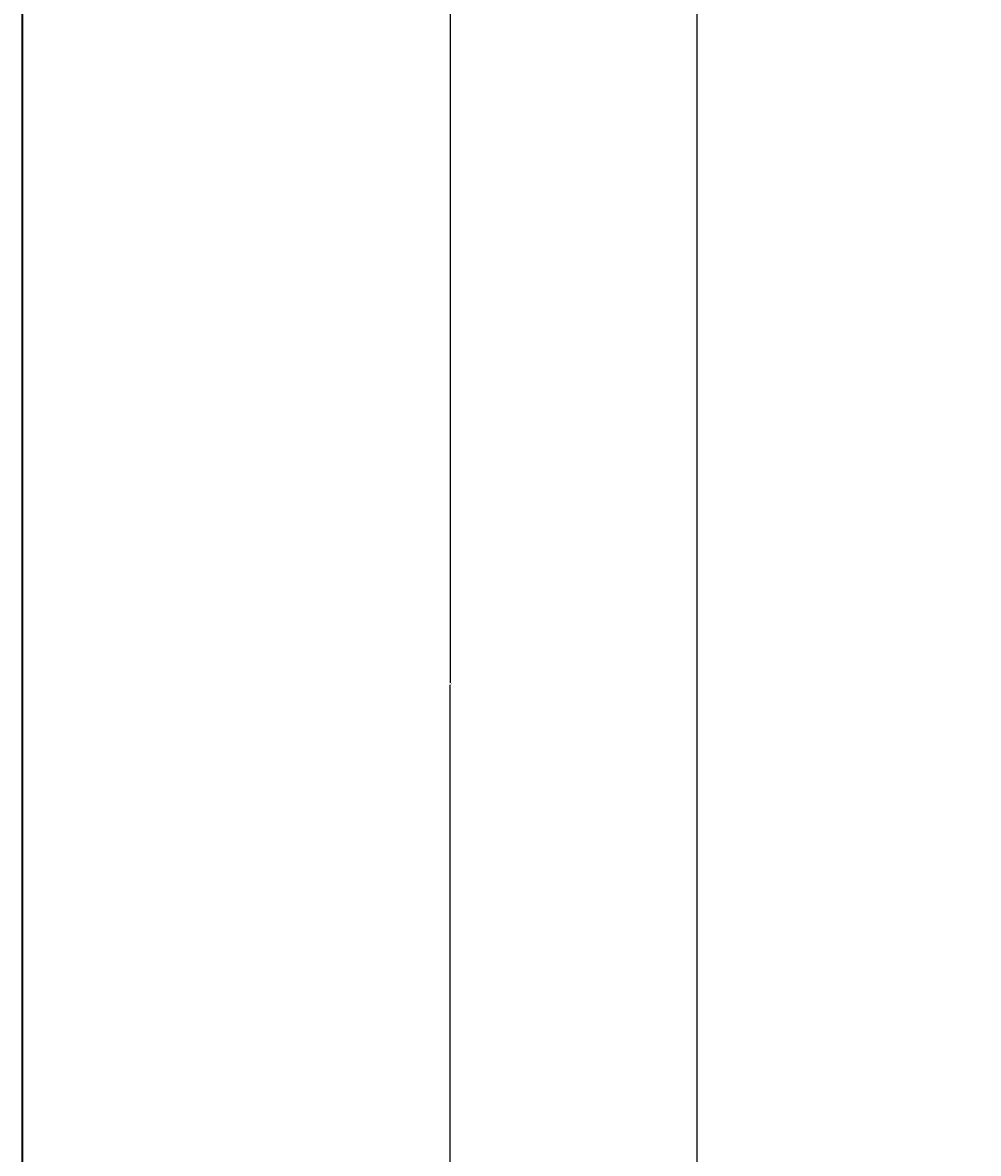
# Model space of a CAD drawing. Units: inches. Extents: x 1824 to 3509, y 619 to 2294.
# Tile 3 of 12: x 1824 to 2001, y 1115 to 1325. Entities that reach past the tile are written whole.
import ezdxf

# ---------------------------------------------------------------- set-up
doc = ezdxf.new("R2010")
doc.units = ezdxf.units.IN
doc.layers.add('A-ANNO-DIMS', color=2, linetype='Continuous', lineweight=18)
doc.layers.add('A-ANNO-TTLB', color=7, linetype='Continuous', lineweight=35)
doc.styles.get("Standard").update_dxf_attribs({"font": 'arial.ttf'})
doc.dimstyles.get("Standard").update_dxf_attribs({"dimtxt": 0.18, "dimasz": 0.18, "dimexe": 0.18, "dimexo": 0.0625, "dimgap": 0.09, "dimtad": 0, "dimtih": 1, "dimtoh": 1, "dimdec": 4, "dimzin": 0, "dimdsep": 46, "dimtxsty": 'Standard', "dimcen": 0.09, "dimadec": 0, "dimazin": 0, "dimtfac": 1, "dimtdec": 4, "dimtofl": 0, "dimtmove": 0, "dimatfit": 3, "dimfxl": 1, "dimtolj": 1, "dimtzin": 0, "dimarcsym": 0})

# ---------------------------------------------------------------- blocks, each defined once
blk = doc.blocks.new('*D94')
at = {"layer": 'A-ANNO-DIMS', "color": 0, "lineweight": -2, "transparency": 16777216}
for p, q in [((1949.09, 1049.16), (1949.09, 1668.03)), ((1949.27, 1667.85), (2235.8, 1667.85)), ((2522.91, 1667.85), (2236.38, 1667.85)), ((2523.09, 1622.16), (2523.09, 1668.03))]:
    blk.add_line(p, q, dxfattribs=at)
at = {"layer": 'A-ANNO-DIMS', "color": 0, "transparency": 16777216}
for points in [[(1949.27, 1667.88), (1949.27, 1667.82), (1949.09, 1667.85)], [(2522.91, 1667.88), (2522.91, 1667.82), (2523.09, 1667.85)]]:
    blk.add_solid(points, dxfattribs=at)
at = {"layer": 'Defpoints', "color": 0, "transparency": 16777216}
for p in [(2523.09, 1667.85), (2523.09, 1622.1), (1949.09, 1049.1)]:
    blk.add_point(p, dxfattribs=at)
at = {"layer": 'A-ANNO-DIMS', "color": 0, "transparency": 16777216, "insert": (2236.09, 1667.85), "char_height": 0.18, "attachment_point": 5}
blk.add_mtext('\\A1;574', dxfattribs=at)
blk = doc.blocks.new('*D95')
at = {"layer": 'A-ANNO-DIMS', "color": 0, "lineweight": -2, "transparency": 16777216}
for p, q in [((2006.03, 1622.1), (1903.16, 1622.1)), ((1903.34, 1621.92), (1903.34, 1202.28)), ((1903.34, 782.28), (1903.34, 1201.92)), ((1949.03, 782.1), (1903.16, 782.1))]:
    blk.add_line(p, q, dxfattribs=at)
at = {"layer": 'A-ANNO-DIMS', "color": 0, "transparency": 16777216}
for points in [[(1903.31, 1621.92), (1903.37, 1621.92), (1903.34, 1622.1)], [(1903.31, 782.28), (1903.37, 782.28), (1903.34, 782.1)]]:
    blk.add_solid(points, dxfattribs=at)
at = {"layer": 'Defpoints', "color": 0, "transparency": 16777216}
for p in [(1903.34, 1622.1), (2006.09, 1622.1), (1949.09, 782.1)]:
    blk.add_point(p, dxfattribs=at)
at = {"layer": 'A-ANNO-DIMS', "color": 0, "transparency": 16777216, "insert": (1903.34, 1202.1), "char_height": 0.18, "attachment_point": 5}
blk.add_mtext('\\A1;840', dxfattribs=at)

msp = doc.modelspace()

# ---------------------------------------------------------------- linework, layer by layer
at = {"layer": 'A-ANNO-TTLB'}
msp.add_lwpolyline([(1824.0608, 2293.6614), (3509.3484, 2293.6614), (3509.3484, 619.4665), (1824.0608, 619.4665)], close=True, dxfattribs=at)

# ---------------------------------------------------------------- dimensions: what is measured, and where the dimension line sits
at = {"layer": 'A-ANNO-DIMS'}
dim = msp.add_linear_dim(base=(2523.0899, 1667.8512), p1=(1949.0899, 1049.1012), p2=(2523.0899, 1622.1012), dimstyle='Standard', override={"dimdec": 0, "dimlfac": 1, "dimrnd": 0, "dimzin": 0, "dimdsep": 46, "dimlunit": 2}, dxfattribs=at)
dim.commit()
dim.dimension.update_dxf_attribs({"geometry": '*D94', "text_midpoint": (2236.0899, 1667.8512)})
dim = msp.add_linear_dim(base=(1903.3399, 1622.1012), p1=(1949.0899, 782.1012), p2=(2006.0899, 1622.1012), angle=90, dimstyle='Standard', override={"dimdec": 0, "dimlfac": 1, "dimrnd": 0, "dimzin": 0, "dimdsep": 46, "dimlunit": 2}, dxfattribs=at)
dim.commit()
dim.dimension.update_dxf_attribs({"geometry": '*D95', "text_midpoint": (1903.3399, 1202.1012)})

doc.saveas('drawing.dxf')
